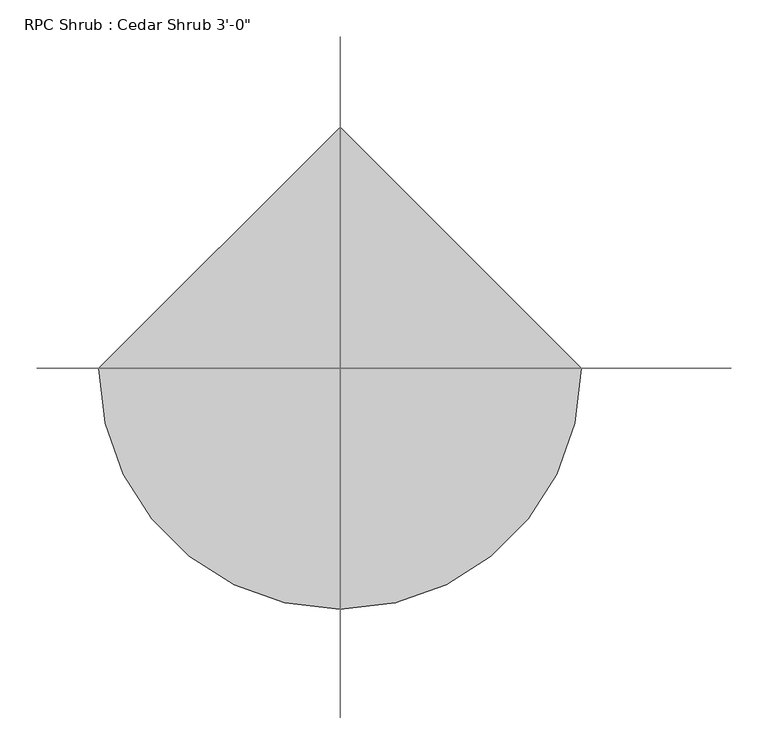
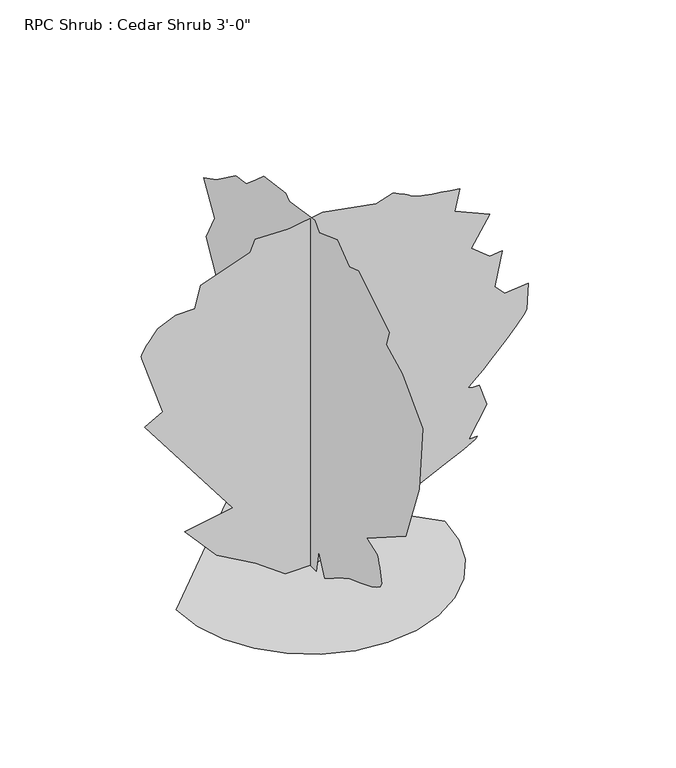
"""IFC4 building model written with IfcOpenShell, lengths in millimetres: geographic element geometry."""

from ifc_helpers import new_model, si_unit, origin, place, context, project, spatial, triangles, source, transform, mapped, element, save


def geographic_element_e27c54a3(model_context):
    return source(origin(), model_context, "Body", "Tessellation", [
        triangles([(-61.9491257, 8.98e-05, 3.1e-06), (-133.3686489, 8.41e-05, 52.0161927), (-229.784339, 7.75e-05, 107.3658847), (-308.3460772, 6.7e-05, 194.8542219), (-190.5039605, 6.45e-05, 216.2798944), (-406.5450977, 3.06e-05, 500.1695792), (-361.9096318, 2.77e-05, 525.1682714), (-413.687576, 9.1e-06, 680.504611), (-414.3708555, 8.5e-06, 686.0316719), (-412.1483531, 7.6e-06, 693.2453304), (-407.5052135, 6.6e-06, 701.8660252), (-400.9240746, 5.4e-06, 711.6120146), (-392.892588, 4.2e-06, 722.1987957), (-383.8933554, 2.8e-06, 733.3493505), (-374.4090142, 1.5e-06, 744.7793941), (-329.7710049, -9e-07, 764.4212185), (-283.347385, -9e-07, 764.4212185), (-269.0649538, -7.7e-06, 821.5560305), (-147.6523519, -1.28e-05, 864.4084293), (-135.1542685, -1.62e-05, 892.975799), (-51.2369207, -1.6e-05, 891.1902248), (30.8950596, -1.77e-05, 905.4726379), (161.2347623, -1.49e-05, 882.2620634), (202.3007514, -1.64e-05, 894.7614458), (209.926594, -1.6e-05, 891.3197227), (217.3964869, -1.56e-05, 887.8932604), (224.5539534, -1.52e-05, 884.4998629), (231.2430618, -1.48e-05, 881.1521021), (237.3073174, -1.44e-05, 877.8678549), (242.5910246, -1.4e-05, 874.6623819), (246.9374708, -1.36e-05, 871.5483278), (253.4703569, -1.33e-05, 868.4368898), (264.8764921, -1.29e-05, 865.2288008), (280.3400286, -1.25e-05, 861.9446262), (299.0547657, -1.21e-05, 858.5968655), (320.205346, -1.17e-05, 855.2034679), (342.9790286, -1.13e-05, 851.779549), (366.5654886, -1.09e-05, 848.337826), (354.0661062, -4.5e-06, 794.774235), (439.7683242, 0.0, 757.2787766), (395.1328583, 8.7e-06, 684.0733612), (439.7683242, 1.3e-05, 648.3660204), (470.1213407, 1.25e-05, 651.9346979), (452.2676702, 2.3e-05, 564.4468695), (477.2638553, 2.59e-05, 539.4507208), (534.3986309, 2.53e-05, 544.8075886), (530.8274099, 3.32e-05, 478.7446515), (523.5757087, 3.45e-05, 467.3451293), (504.7390314, 3.72e-05, 445.2623566), (478.6837177, 4.06e-05, 416.9032228), (449.7886428, 4.42e-05, 386.6696031), (422.4251967, 4.75e-05, 358.9657708), (400.96219, 4.99e-05, 338.196181), (389.7760268, 5.11e-05, 328.7651796), (386.8499336, 5.13e-05, 326.7306381), (386.9235847, 5.15e-05, 325.1634373), (389.4940673, 5.16e-05, 323.9874189), (394.0660629, 5.17e-05, 323.1212654), (400.1341518, 5.18e-05, 322.491362), (407.2029791, 5.19e-05, 322.0189344), (414.7721755, 5.19e-05, 321.622665), (432.6258459, 5.85e-05, 266.2734999), (387.99038, 6.75e-05, 191.2832371), (409.4153077, 6.75e-05, 191.2832371), (404.6121489, 6.81e-05, 185.7135189), (376.0066638, 7e-05, 170.1179047), (327.5713572, 7.28e-05, 146.167468), (263.2661253, 7.65e-05, 115.5335185), (187.0642904, 8.07e-05, 79.8863666), (102.9282468, 8.54e-05, 40.8973356), (14.7802468, 9.02e-05, 3.1e-06), (0.000381, 25.9026863, 6.2e-06), (0.0459126, 34.8300324, 57.3728062), (0.0459011, 134.816453, 119.8644768), (0.045878, 290.1520569, 198.4252067), (0.0458666, 418.7066374, 332.3364006), (0.0458549, 445.4884329, 412.6817508), (0.0458666, 354.4293471, 416.2530081), (0.0458666, 391.9248419, 493.0296444), (0.0458549, 441.9171756, 584.0886938), (0.0458549, 406.2098348, 653.7203447), (0.0458549, 452.6309112, 730.496981), (0.0458549, 400.852967, 757.2787766), (0.0458666, 316.9338161, 817.9848095), (0.0458666, 272.2983865, 825.1272514), (0.0458666, 229.4465145, 860.8371357), (0.045878, 197.3081237, 889.404578), (0.045878, 104.4634274, 901.901417), (0.045878, 90.1794701, 889.404578), (0.0458895, -18.7343943, 907.2582121), (0.0459011, -38.3746062, 885.833357), (0.0459011, -115.1499754, 914.4007267), (0.0459126, -165.1433174, 875.1196215), (0.0459126, -202.6383216, 887.6189312), (0.0459357, -334.7646317, 807.2710739), (0.0459357, -322.2652857, 767.9924395), (0.0459357, -390.1138332, 734.068202), (0.0459474, -477.6016617, 644.7947268), (0.0459588, -463.3167051, 478.7446515), (0.0459474, -404.3962463, 321.622665), (0.0459357, -240.1333076, 216.2798944), (0.0459474, -284.7697909, 200.2108353), (0.0459474, -287.8203315, 191.0282199), (0.0459474, -290.8073766, 181.8458589), (0.0459474, -293.6724997, 172.6634979), (0.0459474, -296.3471184, 163.4808825), (0.0459474, -298.7728243, 154.2985215), (0.0459474, -300.8861037, 145.1161604), (0.0459474, -302.6260048, 135.9335451), (0.0459474, -297.7517384, 125.9028165), (0.0459474, -282.4482212, 114.7161447), (0.0459474, -260.2740114, 103.1860617), (0.0459357, -234.7871223, 92.1246003), (0.0459357, -209.5511809, 82.3433114), (0.0459357, -188.1255083, 74.6549771), (0.0459357, -174.0706613, 69.8711394), (0.0459357, -161.0932739, 63.9628381), (0.0459357, -142.4006376, 53.6509403), (0.0459357, -120.8030006, 40.8714288), (0.0459243, -99.1118918, 27.5610539), (0.0459243, -80.1380772, 15.6561154), (0.0459243, -66.6923272, 7.0931586), (0.0459243, -61.5856531, 3.8085299), (0.0459243, -36.5889844, 59.1581714), (0.0003925, -25.8762707, 0.0), (-329.2655488, 0.0, 9.54e-05), (-320.5609566, -75.445681, 8.64e-05), (-295.7705366, -144.7305826, 7.82e-05), (-256.8780341, -205.8697014, 0.0001171), (-205.8697014, -256.8780341, 0.000111), (-144.7305826, -295.7705366, 0.0001064), (-75.445681, -320.5609566, 0.0001034), (1.15e-05, -329.2655488, 0.0001024), (75.4459354, -320.5609566, 0.0001034), (144.7305826, -295.7705366, 0.0001064), (205.8697014, -256.8780341, 0.000111), (256.8780341, -205.8697014, 0.0001171), (295.7705366, -144.7305826, 7.82e-05), (320.5609566, -75.445681, 8.64e-05), (329.2655488, 2.88e-05, 9.54e-05), (-4.62e-05, 329.2655488, 8.85e-05)], [[63, 64, 65], [63, 65, 66], [3, 4, 5], [42, 43, 44], [45, 46, 47], [5, 6, 7], [39, 40, 41], [37, 38, 39], [2, 3, 5], [45, 47, 48], [45, 48, 49], [36, 37, 39], [60, 61, 62], [19, 20, 21], [59, 60, 62], [59, 62, 63], [58, 59, 63], [57, 58, 63], [56, 57, 63], [45, 49, 50], [17, 18, 19], [35, 36, 39], [45, 50, 51], [44, 45, 51], [44, 51, 52], [41, 42, 44], [23, 24, 25], [34, 35, 39], [44, 52, 53], [41, 44, 53], [41, 53, 54], [41, 54, 55], [1, 2, 5], [71, 1, 5], [70, 71, 5], [69, 70, 5], [68, 69, 5], [68, 5, 7], [67, 68, 7], [66, 67, 7], [63, 66, 7], [56, 63, 7], [55, 56, 7], [41, 55, 7], [39, 41, 7], [34, 39, 7], [33, 34, 7], [32, 33, 7], [31, 32, 7], [30, 31, 7], [29, 30, 7], [28, 29, 7], [27, 28, 7], [26, 27, 7], [25, 26, 7], [23, 25, 7], [22, 23, 7], [21, 22, 7], [19, 21, 7], [17, 19, 7], [17, 7, 8], [16, 17, 8], [15, 16, 8], [14, 15, 8], [13, 14, 8], [12, 13, 8], [11, 12, 8], [10, 11, 8], [9, 10, 8], [76, 77, 78], [122, 123, 124], [81, 82, 83], [121, 122, 124], [124, 125, 72], [124, 72, 73], [75, 76, 78], [120, 121, 124], [94, 95, 96], [93, 94, 96], [91, 92, 93], [119, 120, 124], [89, 90, 91], [79, 80, 81], [101, 102, 103], [81, 83, 84], [81, 84, 85], [97, 98, 99], [87, 88, 89], [96, 97, 99], [74, 75, 78], [96, 99, 100], [96, 100, 101], [93, 96, 101], [91, 93, 101], [89, 91, 101], [87, 89, 101], [86, 87, 101], [85, 86, 101], [81, 85, 101], [79, 81, 101], [78, 79, 101], [74, 78, 101], [73, 74, 101], [124, 73, 101], [119, 124, 101], [118, 119, 101], [117, 118, 101], [116, 117, 101], [115, 116, 101], [114, 115, 101], [113, 114, 101], [112, 113, 101], [112, 101, 103], [112, 103, 104], [112, 104, 105], [111, 112, 105], [111, 105, 106], [111, 106, 107], [110, 111, 107], [110, 107, 108], [109, 110, 108], [140, 141, 126], [139, 140, 126], [139, 126, 127], [138, 139, 127], [138, 127, 128], [138, 128, 129], [137, 138, 129], [136, 137, 129], [136, 129, 130], [136, 130, 131], [136, 131, 132], [136, 132, 133], [136, 133, 134], [136, 134, 135]], closed=False),
    ])


if __name__ == "__main__":
    model = new_model("IFC4")
    model_context = context("Model", 3, world=origin())
    ifc_project = project(units=[si_unit("LENGTHUNIT", "METRE", prefix="MILLI")], contexts=[model_context])
    site = spatial("IfcSite", under=ifc_project)
    building = spatial("IfcBuilding", under=site)
    placement = place(None, origin())
    geographic_element_shape = geographic_element_e27c54a3(model_context)
    element("IfcGeographicElement", 1, ObjectType="RPC Shrub : Cedar Shrub 3'-0\"", at=placement, inside=building, context=model_context, shape_type="MappedRepresentation", body=[
        mapped(geographic_element_shape, transform((0.0, 0.0, 0.0), x_axis=(1.0, 0.0, 0.0), y_axis=(0.0, 1.0, 0.0), z_axis=(0.0, 0.0, 1.0))),
    ])
    save(model, "model.ifc")

# Revit data of these elements
# Type "RPC Shrub : Cedar Shrub 3'-0\""
#   Type Comments = "Cedar Shrub"
#   built-in parameter 1005198 = "{2, 15},{39, RPC-16-FUMD-ULXX-U7X6-J000-ST1L-LVER-AU},{1, 0},{1, 0},{2, 35},{1, 8},{5, Color},{1, 0},{1, 0},{3, 0.8},{3, 0.8},{3, 0.8},{1, 8},{7, BBoxMin},{1, 0},{1, 0},{1, 0},{1, 0},{1, 0},{1, 8},{7, BBoxMax},{1, 0},{1, 0},{1, 0},{1, 0},{1, 0},{2, 11},{9, RPCTypeId},{1, 0},{1, 0},{39, RPC-16-FUMD-ULXX-U7X6-J000-ST1L-LVER-AU},{1, 6},{14, RPCPlantHeight},{1, 0},{1, 0},{1, 3},{2, 11},{7, keyword},{1, 0},{1, 0},{158, :Geometry:RPC:Cedar Shrub:Little Bush:cedar:miniature:evergreen:conifer:shrub:eastern red cedar:juniper:hedge:juniperus virginiana:genevrier de virginie:thuja},{2, 11},{8, category},{1, 0},{1, 0},{17, :Shrubs [General]},{2, 11},{12, LocalizedUID},{1, 0},{1, 0},{11, Cedar Shrub},{2, 14},{6, Height},{1, 0},{1, 0},{1, 3},{1, 2},{16, Cast Reflections},{1, 0},{1, 0},{1, 0},{1, 2},{12, Cast Shadows},{1, 0},{1, 0},{1, 1},{1, 2},{9, Lock View},{1, 0},{1, 0},{1, 0},{1, 4},{5, ViewC},{1, 0},{1, 0},{1, 0},{2, 11},{20, AdvancedUIDefinition},{1, 0},{1, 0},{0, },{2, 11},{10, AssetLibID},{1, 0},{1, 0},{36, 4D3F6E72-3F99-4203-98E9-AF80B3C7A7A4},{2, 11},{10, BaseSchema},{1, 0},{1, 0},{9, RPCSchema},{2, 11},{12, ExchangeGUID},{1, 0},{1, 0},{0, },{1, 2},{6, Hidden},{1, 0},{1, 0},{1, 0},{1, 4},{11, RPCCategory},{1, 0},{1, 0},{1, 0},{2, 11},{8, RPCImage},{1, 0},{1, 0},{0, },{1, 4},{13, SchemaVersion},{1, 0},{1, 0},{1, 4},{2, 11},{12, UIDefinition},{1, 0},{1, 0},{0, },{2, 11},{6, UIName},{1, 0},{1, 0},{39, RPC-16-FUMD-ULXX-U7X6-J000-ST1L-LVER-AU},{2, 11},{11, VersionGUID},{1, 0},{1, 0},{9, RPCSchema},{2, 11},{9, assettype},{1, 0},{1, 0},{11, RPCGeometry},{2, 11},{11, description},{1, 0},{1, 0},{0, },{2, 11},{9, localname},{1, 0},{1, 0},{3, RPC},{2, 11},{9, localtype},{1, 0},{1, 0},{3, RPC},{1, 4},{8, revision},{1, 0},{1, 0},{1, 1},{2, 11},{9, thumbnail},{1, 0},{1, 0},{0, },{1, 4},{7, version},{1, 0},{1, 0},{1, 1},{1, 2},{20, RPC_Cast Reflections},{1, 0},{1, 0},{1, 1},{1, 2},{16, RPC_Cast Shadows},{1, 0},{1, 0},{1, 1},{1, 2},{13, RPC_Lock View},{1, 0},{1, 0},{1, 0},{1, 4},{9, RPC_ViewC},{1, 0},{1, 0},{1, 0},{21, assetlibrary_base.fbx},{1, 5},"
#   built-in parameter 1005195 = "RPC-16-FUMD-ULXX-U7X6-J000-ST1L-LVER-AU"
#   Assembly Code = "G2050500"
#   Height = 3' - 0"
#   Default Elevation = 0
